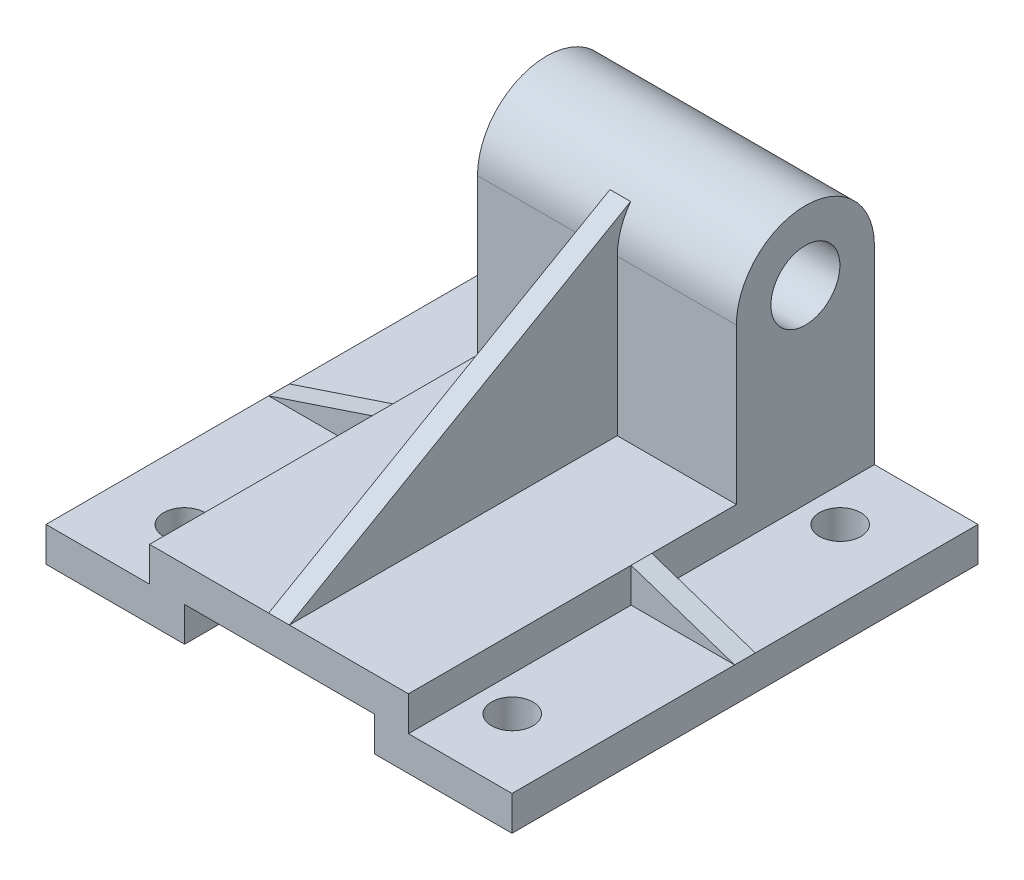
ISO-10303-21;
HEADER;
FILE_DESCRIPTION(('STEP AP214'),'2;1');
FILE_NAME('part.step','',(''),(''),'','','');
FILE_SCHEMA(('AUTOMOTIVE_DESIGN { 1 0 10303 214 1 1 1 1 }'));
ENDSEC;
DATA;
#1=APPLICATION_CONTEXT('core data for automotive mechanical design processes');
#2=APPLICATION_PROTOCOL_DEFINITION('international standard','automotive_design',2000,#1);
#3=PRODUCT_CONTEXT('',#1,'mechanical');
#4=PRODUCT('Part','Part','',(#3));
#5=PRODUCT_RELATED_PRODUCT_CATEGORY('part','',(#4));
#6=PRODUCT_DEFINITION_FORMATION('','',#4);
#7=PRODUCT_DEFINITION_CONTEXT('part definition',#1,'design');
#8=PRODUCT_DEFINITION('design','',#6,#7);
#9=PRODUCT_DEFINITION_SHAPE('','',#8);
#10=(LENGTH_UNIT() NAMED_UNIT(*) SI_UNIT(.MILLI.,.METRE.));
#11=(NAMED_UNIT(*) PLANE_ANGLE_UNIT() SI_UNIT($,.RADIAN.));
#12=(NAMED_UNIT(*) SI_UNIT($,.STERADIAN.) SOLID_ANGLE_UNIT());
#13=UNCERTAINTY_MEASURE_WITH_UNIT(LENGTH_MEASURE(1.E-05),#10,'distance_accuracy_value','');
#14=(GEOMETRIC_REPRESENTATION_CONTEXT(3) GLOBAL_UNCERTAINTY_ASSIGNED_CONTEXT((#13)) GLOBAL_UNIT_ASSIGNED_CONTEXT((#10,
#11,#12)) REPRESENTATION_CONTEXT('',''));
#15=CARTESIAN_POINT('',(0.,0.,0.));
#16=DIRECTION('',(0.,0.,1.));
#17=DIRECTION('',(1.,0.,0.));
#18=AXIS2_PLACEMENT_3D('',#15,#16,#17);
#19=CARTESIAN_POINT('',(-67.5,10.,67.5));
#20=DIRECTION('',(0.,-1.,0.));
#21=DIRECTION('',(0.,0.,-1.));
#22=AXIS2_PLACEMENT_3D('',#19,#20,#21);
#23=PLANE('',#22);
#24=DIRECTION('',(0.,0.,-1.));
#25=VECTOR('',#24,1.);
#26=CARTESIAN_POINT('',(-3.,10.,-35.5000326124525));
#27=LINE('',#26,#25);
#28=CARTESIAN_POINT('',(-3.,10.,67.5));
#29=VERTEX_POINT('',#28);
#30=CARTESIAN_POINT('',(-3.,10.,-27.5));
#31=VERTEX_POINT('',#30);
#32=EDGE_CURVE('E288',#29,#31,#27,.T.);
#33=ORIENTED_EDGE('',*,*,#32,.T.);
#34=DIRECTION('',(1.,0.,0.));
#35=VECTOR('',#34,1.);
#36=CARTESIAN_POINT('',(-37.5,10.,-27.5));
#37=LINE('',#36,#35);
#38=CARTESIAN_POINT('',(-37.5,10.,-27.5));
#39=VERTEX_POINT('',#38);
#40=EDGE_CURVE('E358',#39,#31,#37,.T.);
#41=ORIENTED_EDGE('',*,*,#40,.F.);
#42=DIRECTION('',(0.,0.,1.));
#43=VECTOR('',#42,1.);
#44=CARTESIAN_POINT('',(-37.5,10.,-67.5));
#45=LINE('',#44,#43);
#46=CARTESIAN_POINT('',(-37.5,10.,-3.));
#47=VERTEX_POINT('',#46);
#48=EDGE_CURVE('E382',#39,#47,#45,.T.);
#49=ORIENTED_EDGE('',*,*,#48,.T.);
#50=DIRECTION('',(0.,0.,-1.));
#51=VECTOR('',#50,1.);
#52=CARTESIAN_POINT('',(-37.5,10.,3.));
#53=LINE('',#52,#51);
#54=CARTESIAN_POINT('',(-37.5,10.,3.));
#55=VERTEX_POINT('',#54);
#56=EDGE_CURVE('E332',#55,#47,#53,.T.);
#57=ORIENTED_EDGE('',*,*,#56,.F.);
#58=CARTESIAN_POINT('',(-37.5,10.,67.5));
#59=VERTEX_POINT('',#58);
#60=EDGE_CURVE('E381',#55,#59,#45,.T.);
#61=ORIENTED_EDGE('',*,*,#60,.T.);
#62=DIRECTION('',(-1.,0.,0.));
#63=VECTOR('',#62,1.);
#64=CARTESIAN_POINT('',(-67.5,10.,67.5));
#65=LINE('',#64,#63);
#66=EDGE_CURVE('E232',#29,#59,#65,.T.);
#67=ORIENTED_EDGE('',*,*,#66,.F.);
#68=EDGE_LOOP('',(#33,#41,#49,#57,#61,#67));
#69=FACE_BOUND('',#68,.T.);
#70=ADVANCED_FACE('F41',(#69),#23,.F.);
#71=CARTESIAN_POINT('',(-37.5,55.,-27.5));
#72=DIRECTION('',(0.,0.,1.));
#73=DIRECTION('',(1.,0.,0.));
#74=AXIS2_PLACEMENT_3D('',#71,#72,#73);
#75=PLANE('',#74);
#76=ORIENTED_EDGE('',*,*,#40,.T.);
#77=DIRECTION('',(0.,1.,0.));
#78=VECTOR('',#77,1.);
#79=CARTESIAN_POINT('',(-3.,55.,-27.5));
#80=LINE('',#79,#78);
#81=CARTESIAN_POINT('',(-3.,55.,-27.5));
#82=VERTEX_POINT('',#81);
#83=EDGE_CURVE('E220',#31,#82,#80,.T.);
#84=ORIENTED_EDGE('',*,*,#83,.T.);
#85=DIRECTION('',(1.,0.,0.));
#86=VECTOR('',#85,1.);
#87=CARTESIAN_POINT('',(-37.5,55.,-27.5));
#88=LINE('',#87,#86);
#89=CARTESIAN_POINT('',(-37.5,55.,-27.5));
#90=VERTEX_POINT('',#89);
#91=EDGE_CURVE('E360',#90,#82,#88,.T.);
#92=ORIENTED_EDGE('',*,*,#91,.F.);
#93=DIRECTION('',(0.,-1.,0.));
#94=VECTOR('',#93,1.);
#95=CARTESIAN_POINT('',(-37.5,55.,-27.5));
#96=LINE('',#95,#94);
#97=EDGE_CURVE('E346',#90,#39,#96,.T.);
#98=ORIENTED_EDGE('',*,*,#97,.T.);
#99=EDGE_LOOP('',(#76,#84,#92,#98));
#100=FACE_BOUND('',#99,.T.);
#101=ADVANCED_FACE('F488',(#100),#75,.T.);
#102=CARTESIAN_POINT('',(37.5,0.,-67.5));
#103=DIRECTION('',(-1.,0.,0.));
#104=DIRECTION('',(0.,0.,1.));
#105=AXIS2_PLACEMENT_3D('',#102,#103,#104);
#106=PLANE('',#105);
#107=CARTESIAN_POINT('',(37.5,55.,-47.5));
#108=DIRECTION('',(1.,0.,0.));
#109=DIRECTION('',(0.,0.,-1.));
#110=AXIS2_PLACEMENT_3D('',#107,#108,#109);
#111=CIRCLE('',#110,10.);
#112=CARTESIAN_POINT('',(37.5,55.,-57.5));
#113=VERTEX_POINT('',#112);
#114=EDGE_CURVE('E340',#113,#113,#111,.T.);
#115=ORIENTED_EDGE('',*,*,#114,.F.);
#116=EDGE_LOOP('',(#115));
#117=FACE_BOUND('',#116,.T.);
#118=DIRECTION('',(0.,1.,0.));
#119=VECTOR('',#118,1.);
#120=CARTESIAN_POINT('',(37.5,10.,-3.));
#121=LINE('',#120,#119);
#122=CARTESIAN_POINT('',(37.5,0.,-3.));
#123=VERTEX_POINT('',#122);
#124=CARTESIAN_POINT('',(37.5,10.,-3.));
#125=VERTEX_POINT('',#124);
#126=EDGE_CURVE('E301',#123,#125,#121,.T.);
#127=ORIENTED_EDGE('',*,*,#126,.F.);
#128=DIRECTION('',(0.,0.,1.));
#129=VECTOR('',#128,1.);
#130=CARTESIAN_POINT('',(37.5,0.,-67.5));
#131=LINE('',#130,#129);
#132=CARTESIAN_POINT('',(37.5,0.,-67.5));
#133=VERTEX_POINT('',#132);
#134=EDGE_CURVE('E407',#133,#123,#131,.T.);
#135=ORIENTED_EDGE('',*,*,#134,.F.);
#136=DIRECTION('',(0.,-1.,0.));
#137=VECTOR('',#136,1.);
#138=CARTESIAN_POINT('',(37.5,0.,-67.5));
#139=LINE('',#138,#137);
#140=CARTESIAN_POINT('',(37.5,55.,-67.5));
#141=VERTEX_POINT('',#140);
#142=EDGE_CURVE('E389',#141,#133,#139,.T.);
#143=ORIENTED_EDGE('',*,*,#142,.F.);
#144=CARTESIAN_POINT('',(37.5,55.,-47.5));
#145=DIRECTION('',(1.,0.,0.));
#146=DIRECTION('',(0.,0.,-1.));
#147=AXIS2_PLACEMENT_3D('',#144,#145,#146);
#148=CIRCLE('',#147,20.);
#149=CARTESIAN_POINT('',(37.5,55.,-27.5));
#150=VERTEX_POINT('',#149);
#151=EDGE_CURVE('E342',#141,#150,#148,.T.);
#152=ORIENTED_EDGE('',*,*,#151,.T.);
#153=DIRECTION('',(0.,-1.,0.));
#154=VECTOR('',#153,1.);
#155=CARTESIAN_POINT('',(37.5,55.,-27.5));
#156=LINE('',#155,#154);
#157=CARTESIAN_POINT('',(37.5,10.,-27.5));
#158=VERTEX_POINT('',#157);
#159=EDGE_CURVE('E350',#150,#158,#156,.T.);
#160=ORIENTED_EDGE('',*,*,#159,.T.);
#161=DIRECTION('',(0.,0.,1.));
#162=VECTOR('',#161,1.);
#163=CARTESIAN_POINT('',(37.5,10.,-67.5));
#164=LINE('',#163,#162);
#165=EDGE_CURVE('E372',#158,#125,#164,.T.);
#166=ORIENTED_EDGE('',*,*,#165,.T.);
#167=EDGE_LOOP('',(#127,#135,#143,#152,#160,#166));
#168=FACE_BOUND('',#167,.T.);
#169=ADVANCED_FACE('F493',(#117,#168),#106,.F.);
#170=CARTESIAN_POINT('',(0.,0.,-67.5));
#171=DIRECTION('',(0.,-1.,0.));
#172=DIRECTION('',(0.,0.,-1.));
#173=AXIS2_PLACEMENT_3D('',#170,#171,#172);
#174=PLANE('',#173);
#175=CARTESIAN_POINT('',(47.5715920769878,0.,-47.5));
#176=DIRECTION('',(0.,-1.,0.));
#177=DIRECTION('',(0.,0.,-1.));
#178=AXIS2_PLACEMENT_3D('',#175,#176,#177);
#179=CIRCLE('',#178,6.);
#180=CARTESIAN_POINT('',(47.5715920769878,0.,-53.5));
#181=VERTEX_POINT('',#180);
#182=EDGE_CURVE('E286',#181,#181,#179,.T.);
#183=ORIENTED_EDGE('',*,*,#182,.T.);
#184=EDGE_LOOP('',(#183));
#185=FACE_BOUND('',#184,.T.);
#186=DIRECTION('',(-1.,0.,0.));
#187=VECTOR('',#186,1.);
#188=CARTESIAN_POINT('',(37.5,0.,-3.));
#189=LINE('',#188,#187);
#190=CARTESIAN_POINT('',(67.5000000000001,0.,-3.));
#191=VERTEX_POINT('',#190);
#192=EDGE_CURVE('E300',#191,#123,#189,.T.);
#193=ORIENTED_EDGE('',*,*,#192,.F.);
#194=DIRECTION('',(0.,0.,1.));
#195=VECTOR('',#194,1.);
#196=CARTESIAN_POINT('',(67.5000000000001,0.,-67.5));
#197=LINE('',#196,#195);
#198=CARTESIAN_POINT('',(67.5000000000001,0.,-67.5));
#199=VERTEX_POINT('',#198);
#200=EDGE_CURVE('E405',#199,#191,#197,.T.);
#201=ORIENTED_EDGE('',*,*,#200,.F.);
#202=DIRECTION('',(1.,0.,0.));
#203=VECTOR('',#202,1.);
#204=CARTESIAN_POINT('',(0.,0.,-67.5));
#205=LINE('',#204,#203);
#206=EDGE_CURVE('E394',#133,#199,#205,.T.);
#207=ORIENTED_EDGE('',*,*,#206,.F.);
#208=ORIENTED_EDGE('',*,*,#134,.T.);
#209=EDGE_LOOP('',(#193,#201,#207,#208));
#210=FACE_BOUND('',#209,.T.);
#211=ADVANCED_FACE('F514',(#185,#210),#174,.F.);
#212=CARTESIAN_POINT('',(0.,0.,-67.5));
#213=DIRECTION('',(0.,1.,0.));
#214=DIRECTION('',(0.,0.,1.));
#215=AXIS2_PLACEMENT_3D('',#212,#213,#214);
#216=PLANE('',#215);
#217=CARTESIAN_POINT('',(-47.4284079230122,0.,-47.5));
#218=DIRECTION('',(0.,1.,0.));
#219=DIRECTION('',(0.,0.,1.));
#220=AXIS2_PLACEMENT_3D('',#217,#218,#219);
#221=CIRCLE('',#220,6.);
#222=CARTESIAN_POINT('',(-47.4284079230122,0.,-41.5));
#223=VERTEX_POINT('',#222);
#224=EDGE_CURVE('E272',#223,#223,#221,.T.);
#225=ORIENTED_EDGE('',*,*,#224,.F.);
#226=EDGE_LOOP('',(#225));
#227=FACE_BOUND('',#226,.T.);
#228=DIRECTION('',(0.,0.,1.));
#229=VECTOR('',#228,1.);
#230=CARTESIAN_POINT('',(-67.5,0.,-67.5));
#231=LINE('',#230,#229);
#232=CARTESIAN_POINT('',(-67.5,0.,-67.5));
#233=VERTEX_POINT('',#232);
#234=CARTESIAN_POINT('',(-67.5,0.,-3.));
#235=VERTEX_POINT('',#234);
#236=EDGE_CURVE('E376',#233,#235,#231,.T.);
#237=ORIENTED_EDGE('',*,*,#236,.T.);
#238=DIRECTION('',(1.,0.,0.));
#239=VECTOR('',#238,1.);
#240=CARTESIAN_POINT('',(-37.5,0.,-3.));
#241=LINE('',#240,#239);
#242=CARTESIAN_POINT('',(-37.5,0.,-3.));
#243=VERTEX_POINT('',#242);
#244=EDGE_CURVE('E320',#235,#243,#241,.T.);
#245=ORIENTED_EDGE('',*,*,#244,.T.);
#246=DIRECTION('',(0.,0.,1.));
#247=VECTOR('',#246,1.);
#248=CARTESIAN_POINT('',(-37.5,0.,-67.5));
#249=LINE('',#248,#247);
#250=CARTESIAN_POINT('',(-37.5,0.,-67.5));
#251=VERTEX_POINT('',#250);
#252=EDGE_CURVE('E383',#251,#243,#249,.T.);
#253=ORIENTED_EDGE('',*,*,#252,.F.);
#254=DIRECTION('',(-1.,0.,0.));
#255=VECTOR('',#254,1.);
#256=CARTESIAN_POINT('',(0.,0.,-67.5));
#257=LINE('',#256,#255);
#258=EDGE_CURVE('E362',#251,#233,#257,.T.);
#259=ORIENTED_EDGE('',*,*,#258,.T.);
#260=EDGE_LOOP('',(#237,#245,#253,#259));
#261=FACE_BOUND('',#260,.T.);
#262=ADVANCED_FACE('F504',(#227,#261),#216,.T.);
#263=CARTESIAN_POINT('',(-37.5,0.,-67.5));
#264=DIRECTION('',(-1.,0.,0.));
#265=DIRECTION('',(0.,0.,1.));
#266=AXIS2_PLACEMENT_3D('',#263,#264,#265);
#267=PLANE('',#266);
#268=CARTESIAN_POINT('',(-37.5,55.,-47.5));
#269=DIRECTION('',(1.,0.,0.));
#270=DIRECTION('',(0.,0.,-1.));
#271=AXIS2_PLACEMENT_3D('',#268,#269,#270);
#272=CIRCLE('',#271,10.);
#273=CARTESIAN_POINT('',(-37.5,55.,-57.5));
#274=VERTEX_POINT('',#273);
#275=EDGE_CURVE('E336',#274,#274,#272,.T.);
#276=ORIENTED_EDGE('',*,*,#275,.T.);
#277=EDGE_LOOP('',(#276));
#278=FACE_BOUND('',#277,.T.);
#279=ORIENTED_EDGE('',*,*,#252,.T.);
#280=DIRECTION('',(0.,1.,0.));
#281=VECTOR('',#280,1.);
#282=CARTESIAN_POINT('',(-37.5,10.,-3.));
#283=LINE('',#282,#281);
#284=EDGE_CURVE('E330',#243,#47,#283,.T.);
#285=ORIENTED_EDGE('',*,*,#284,.T.);
#286=ORIENTED_EDGE('',*,*,#48,.F.);
#287=ORIENTED_EDGE('',*,*,#97,.F.);
#288=CARTESIAN_POINT('',(-37.5,55.,-47.5));
#289=DIRECTION('',(1.,0.,0.));
#290=DIRECTION('',(0.,0.,-1.));
#291=AXIS2_PLACEMENT_3D('',#288,#289,#290);
#292=CIRCLE('',#291,20.);
#293=CARTESIAN_POINT('',(-37.5,55.,-67.5));
#294=VERTEX_POINT('',#293);
#295=EDGE_CURVE('E341',#294,#90,#292,.T.);
#296=ORIENTED_EDGE('',*,*,#295,.F.);
#297=DIRECTION('',(0.,-1.,0.));
#298=VECTOR('',#297,1.);
#299=CARTESIAN_POINT('',(-37.5,0.,-67.5));
#300=LINE('',#299,#298);
#301=EDGE_CURVE('E370',#294,#251,#300,.T.);
#302=ORIENTED_EDGE('',*,*,#301,.T.);
#303=EDGE_LOOP('',(#279,#285,#286,#287,#296,#302));
#304=FACE_BOUND('',#303,.T.);
#305=ADVANCED_FACE('F498',(#278,#304),#267,.T.);
#306=CARTESIAN_POINT('',(3.,10.,-27.5));
#307=VERTEX_POINT('',#306);
#308=EDGE_CURVE('E228',#307,#158,#37,.T.);
#309=ORIENTED_EDGE('',*,*,#308,.F.);
#310=DIRECTION('',(0.,0.,-1.));
#311=VECTOR('',#310,1.);
#312=CARTESIAN_POINT('',(3.,10.,-29.4496870036438));
#313=LINE('',#312,#311);
#314=CARTESIAN_POINT('',(3.,10.,67.5));
#315=VERTEX_POINT('',#314);
#316=EDGE_CURVE('E210',#315,#307,#313,.T.);
#317=ORIENTED_EDGE('',*,*,#316,.F.);
#318=CARTESIAN_POINT('',(37.5,10.,67.5));
#319=VERTEX_POINT('',#318);
#320=EDGE_CURVE('E222',#319,#315,#65,.T.);
#321=ORIENTED_EDGE('',*,*,#320,.F.);
#322=CARTESIAN_POINT('',(37.5,10.,3.));
#323=VERTEX_POINT('',#322);
#324=EDGE_CURVE('E402',#323,#319,#164,.T.);
#325=ORIENTED_EDGE('',*,*,#324,.F.);
#326=DIRECTION('',(0.,0.,-1.));
#327=VECTOR('',#326,1.);
#328=CARTESIAN_POINT('',(37.5,10.,3.));
#329=LINE('',#328,#327);
#330=EDGE_CURVE('E304',#323,#125,#329,.T.);
#331=ORIENTED_EDGE('',*,*,#330,.T.);
#332=ORIENTED_EDGE('',*,*,#165,.F.);
#333=EDGE_LOOP('',(#309,#317,#321,#325,#331,#332));
#334=FACE_BOUND('',#333,.T.);
#335=ADVANCED_FACE('F223',(#334),#23,.F.);
#336=CARTESIAN_POINT('',(-67.5,10.,67.5));
#337=DIRECTION('',(1.,0.,0.));
#338=DIRECTION('',(0.,1.,0.));
#339=AXIS2_PLACEMENT_3D('',#336,#337,#338);
#340=PLANE('',#339);
#341=ORIENTED_EDGE('',*,*,#236,.F.);
#342=DIRECTION('',(0.,-1.,0.));
#343=VECTOR('',#342,1.);
#344=CARTESIAN_POINT('',(-67.5,10.,-67.5));
#345=LINE('',#344,#343);
#346=CARTESIAN_POINT('',(-67.4999999999999,-10.,-67.5));
#347=VERTEX_POINT('',#346);
#348=EDGE_CURVE('E249',#233,#347,#345,.T.);
#349=ORIENTED_EDGE('',*,*,#348,.T.);
#350=DIRECTION('',(0.,0.,-1.));
#351=VECTOR('',#350,1.);
#352=CARTESIAN_POINT('',(-67.4999999999999,-10.,67.5));
#353=LINE('',#352,#351);
#354=CARTESIAN_POINT('',(-67.4999999999999,-10.,67.5));
#355=VERTEX_POINT('',#354);
#356=EDGE_CURVE('E256',#355,#347,#353,.T.);
#357=ORIENTED_EDGE('',*,*,#356,.F.);
#358=DIRECTION('',(0.,-1.,0.));
#359=VECTOR('',#358,1.);
#360=CARTESIAN_POINT('',(-67.5,10.,67.5));
#361=LINE('',#360,#359);
#362=CARTESIAN_POINT('',(-67.5,0.,67.5));
#363=VERTEX_POINT('',#362);
#364=EDGE_CURVE('E234',#363,#355,#361,.T.);
#365=ORIENTED_EDGE('',*,*,#364,.F.);
#366=CARTESIAN_POINT('',(-67.5,0.,3.));
#367=VERTEX_POINT('',#366);
#368=EDGE_CURVE('E379',#367,#363,#231,.T.);
#369=ORIENTED_EDGE('',*,*,#368,.F.);
#370=DIRECTION('',(0.,0.,-1.));
#371=VECTOR('',#370,1.);
#372=CARTESIAN_POINT('',(-67.5,0.,3.));
#373=LINE('',#372,#371);
#374=EDGE_CURVE('E323',#367,#235,#373,.T.);
#375=ORIENTED_EDGE('',*,*,#374,.T.);
#376=EDGE_LOOP('',(#341,#349,#357,#365,#369,#375));
#377=FACE_BOUND('',#376,.T.);
#378=ADVANCED_FACE('F500',(#377),#340,.F.);
#379=CARTESIAN_POINT('',(0.,0.,67.5));
#380=DIRECTION('',(0.,0.,1.));
#381=DIRECTION('',(1.,0.,0.));
#382=AXIS2_PLACEMENT_3D('',#379,#380,#381);
#383=PLANE('',#382);
#384=DIRECTION('',(0.,-1.,0.));
#385=VECTOR('',#384,1.);
#386=CARTESIAN_POINT('',(-37.5,0.,67.5));
#387=LINE('',#386,#385);
#388=CARTESIAN_POINT('',(-37.5,0.,67.5));
#389=VERTEX_POINT('',#388);
#390=EDGE_CURVE('E368',#59,#389,#387,.T.);
#391=ORIENTED_EDGE('',*,*,#390,.T.);
#392=DIRECTION('',(-1.,0.,0.));
#393=VECTOR('',#392,1.);
#394=CARTESIAN_POINT('',(0.,0.,67.5));
#395=LINE('',#394,#393);
#396=EDGE_CURVE('E371',#389,#363,#395,.T.);
#397=ORIENTED_EDGE('',*,*,#396,.T.);
#398=ORIENTED_EDGE('',*,*,#364,.T.);
#399=DIRECTION('',(1.,0.,0.));
#400=VECTOR('',#399,1.);
#401=CARTESIAN_POINT('',(-67.4999999999999,-10.,67.5));
#402=LINE('',#401,#400);
#403=CARTESIAN_POINT('',(-27.3568158460245,-10.,67.5));
#404=VERTEX_POINT('',#403);
#405=EDGE_CURVE('E243',#355,#404,#402,.T.);
#406=ORIENTED_EDGE('',*,*,#405,.T.);
#407=DIRECTION('',(0.,-1.,0.));
#408=VECTOR('',#407,1.);
#409=CARTESIAN_POINT('',(-27.3568158460245,0.,67.5));
#410=LINE('',#409,#408);
#411=CARTESIAN_POINT('',(-27.3568158460245,0.,67.5));
#412=VERTEX_POINT('',#411);
#413=EDGE_CURVE('E378',#412,#404,#410,.T.);
#414=ORIENTED_EDGE('',*,*,#413,.F.);
#415=DIRECTION('',(-1.,0.,0.));
#416=VECTOR('',#415,1.);
#417=CARTESIAN_POINT('',(27.6431841539755,0.,67.5));
#418=LINE('',#417,#416);
#419=CARTESIAN_POINT('',(27.6431841539755,0.,67.5));
#420=VERTEX_POINT('',#419);
#421=EDGE_CURVE('E411',#420,#412,#418,.T.);
#422=ORIENTED_EDGE('',*,*,#421,.F.);
#423=DIRECTION('',(0.,1.,0.));
#424=VECTOR('',#423,1.);
#425=CARTESIAN_POINT('',(27.6431841539755,-10.,67.5));
#426=LINE('',#425,#424);
#427=CARTESIAN_POINT('',(27.6431841539755,-10.,67.5));
#428=VERTEX_POINT('',#427);
#429=EDGE_CURVE('E419',#428,#420,#426,.T.);
#430=ORIENTED_EDGE('',*,*,#429,.F.);
#431=CARTESIAN_POINT('',(67.5000000000001,-10.,67.5));
#432=VERTEX_POINT('',#431);
#433=EDGE_CURVE('E240',#428,#432,#402,.T.);
#434=ORIENTED_EDGE('',*,*,#433,.T.);
#435=DIRECTION('',(0.,1.,0.));
#436=VECTOR('',#435,1.);
#437=CARTESIAN_POINT('',(67.5000000000001,10.,67.5));
#438=LINE('',#437,#436);
#439=CARTESIAN_POINT('',(67.5000000000001,0.,67.5));
#440=VERTEX_POINT('',#439);
#441=EDGE_CURVE('E237',#432,#440,#438,.T.);
#442=ORIENTED_EDGE('',*,*,#441,.T.);
#443=DIRECTION('',(1.,0.,0.));
#444=VECTOR('',#443,1.);
#445=CARTESIAN_POINT('',(0.,0.,67.5));
#446=LINE('',#445,#444);
#447=CARTESIAN_POINT('',(37.5,0.,67.5));
#448=VERTEX_POINT('',#447);
#449=EDGE_CURVE('E391',#448,#440,#446,.T.);
#450=ORIENTED_EDGE('',*,*,#449,.F.);
#451=DIRECTION('',(0.,-1.,0.));
#452=VECTOR('',#451,1.);
#453=CARTESIAN_POINT('',(37.5,0.,67.5));
#454=LINE('',#453,#452);
#455=EDGE_CURVE('E231',#319,#448,#454,.T.);
#456=ORIENTED_EDGE('',*,*,#455,.F.);
#457=ORIENTED_EDGE('',*,*,#320,.T.);
#458=DIRECTION('',(-1.,0.,0.));
#459=VECTOR('',#458,1.);
#460=CARTESIAN_POINT('',(3.,10.,67.5));
#461=LINE('',#460,#459);
#462=EDGE_CURVE('E215',#315,#29,#461,.T.);
#463=ORIENTED_EDGE('',*,*,#462,.T.);
#464=ORIENTED_EDGE('',*,*,#66,.T.);
#465=EDGE_LOOP('',(#391,#397,#398,#406,#414,#422,#430,#434,#442,#450,#456,#457,#463,#464));
#466=FACE_BOUND('',#465,.T.);
#467=ADVANCED_FACE('F229',(#466),#383,.T.);
#468=CARTESIAN_POINT('',(0.,0.,-67.5));
#469=DIRECTION('',(0.,0.,1.));
#470=DIRECTION('',(1.,0.,0.));
#471=AXIS2_PLACEMENT_3D('',#468,#469,#470);
#472=PLANE('',#471);
#473=ORIENTED_EDGE('',*,*,#258,.F.);
#474=ORIENTED_EDGE('',*,*,#301,.F.);
#475=DIRECTION('',(1.,0.,0.));
#476=VECTOR('',#475,1.);
#477=CARTESIAN_POINT('',(-37.5,55.,-67.5));
#478=LINE('',#477,#476);
#479=EDGE_CURVE('E351',#294,#141,#478,.T.);
#480=ORIENTED_EDGE('',*,*,#479,.T.);
#481=ORIENTED_EDGE('',*,*,#142,.T.);
#482=ORIENTED_EDGE('',*,*,#206,.T.);
#483=DIRECTION('',(0.,1.,0.));
#484=VECTOR('',#483,1.);
#485=CARTESIAN_POINT('',(67.5000000000001,10.,-67.5));
#486=LINE('',#485,#484);
#487=CARTESIAN_POINT('',(67.5000000000001,-10.,-67.5));
#488=VERTEX_POINT('',#487);
#489=EDGE_CURVE('E250',#488,#199,#486,.T.);
#490=ORIENTED_EDGE('',*,*,#489,.F.);
#491=DIRECTION('',(1.,0.,0.));
#492=VECTOR('',#491,1.);
#493=CARTESIAN_POINT('',(-67.4999999999999,-10.,-67.5));
#494=LINE('',#493,#492);
#495=CARTESIAN_POINT('',(27.6431841539755,-10.,-67.5));
#496=VERTEX_POINT('',#495);
#497=EDGE_CURVE('E254',#496,#488,#494,.T.);
#498=ORIENTED_EDGE('',*,*,#497,.F.);
#499=DIRECTION('',(0.,1.,0.));
#500=VECTOR('',#499,1.);
#501=CARTESIAN_POINT('',(27.6431841539755,-10.,-67.5));
#502=LINE('',#501,#500);
#503=CARTESIAN_POINT('',(27.6431841539755,0.,-67.5));
#504=VERTEX_POINT('',#503);
#505=EDGE_CURVE('E412',#496,#504,#502,.T.);
#506=ORIENTED_EDGE('',*,*,#505,.T.);
#507=DIRECTION('',(-1.,0.,0.));
#508=VECTOR('',#507,1.);
#509=CARTESIAN_POINT('',(0.,0.,-67.5));
#510=LINE('',#509,#508);
#511=CARTESIAN_POINT('',(-27.3568158460245,0.,-67.5));
#512=VERTEX_POINT('',#511);
#513=EDGE_CURVE('E409',#504,#512,#510,.T.);
#514=ORIENTED_EDGE('',*,*,#513,.T.);
#515=DIRECTION('',(0.,-1.,0.));
#516=VECTOR('',#515,1.);
#517=CARTESIAN_POINT('',(-27.3568158460245,0.,-67.5));
#518=LINE('',#517,#516);
#519=CARTESIAN_POINT('',(-27.3568158460245,-10.,-67.5));
#520=VERTEX_POINT('',#519);
#521=EDGE_CURVE('E414',#512,#520,#518,.T.);
#522=ORIENTED_EDGE('',*,*,#521,.T.);
#523=EDGE_CURVE('E251',#347,#520,#494,.T.);
#524=ORIENTED_EDGE('',*,*,#523,.F.);
#525=ORIENTED_EDGE('',*,*,#348,.F.);
#526=EDGE_LOOP('',(#473,#474,#480,#481,#482,#490,#498,#506,#514,#522,#524,#525));
#527=FACE_BOUND('',#526,.T.);
#528=ADVANCED_FACE('F444',(#527),#472,.F.);
#529=CARTESIAN_POINT('',(-67.4999999999999,-10.,67.5));
#530=DIRECTION('',(0.,1.,0.));
#531=DIRECTION('',(0.,0.,1.));
#532=AXIS2_PLACEMENT_3D('',#529,#530,#531);
#533=PLANE('',#532);
#534=CARTESIAN_POINT('',(47.5715920769878,-10.,47.5));
#535=DIRECTION('',(0.,-1.,0.));
#536=DIRECTION('',(0.,0.,-1.));
#537=AXIS2_PLACEMENT_3D('',#534,#535,#536);
#538=CIRCLE('',#537,6.);
#539=CARTESIAN_POINT('',(47.5715920769878,-10.,41.5));
#540=VERTEX_POINT('',#539);
#541=EDGE_CURVE('E281',#540,#540,#538,.T.);
#542=ORIENTED_EDGE('',*,*,#541,.F.);
#543=EDGE_LOOP('',(#542));
#544=FACE_BOUND('',#543,.T.);
#545=CARTESIAN_POINT('',(47.5715920769878,-10.,-47.5));
#546=DIRECTION('',(0.,-1.,0.));
#547=DIRECTION('',(0.,0.,-1.));
#548=AXIS2_PLACEMENT_3D('',#545,#546,#547);
#549=CIRCLE('',#548,6.);
#550=CARTESIAN_POINT('',(47.5715920769878,-10.,-53.5));
#551=VERTEX_POINT('',#550);
#552=EDGE_CURVE('E270',#551,#551,#549,.T.);
#553=ORIENTED_EDGE('',*,*,#552,.F.);
#554=EDGE_LOOP('',(#553));
#555=FACE_BOUND('',#554,.T.);
#556=ORIENTED_EDGE('',*,*,#433,.F.);
#557=DIRECTION('',(0.,0.,1.));
#558=VECTOR('',#557,1.);
#559=CARTESIAN_POINT('',(27.6431841539755,-10.,-67.5));
#560=LINE('',#559,#558);
#561=EDGE_CURVE('E424',#496,#428,#560,.T.);
#562=ORIENTED_EDGE('',*,*,#561,.F.);
#563=ORIENTED_EDGE('',*,*,#497,.T.);
#564=DIRECTION('',(0.,0.,-1.));
#565=VECTOR('',#564,1.);
#566=CARTESIAN_POINT('',(67.5000000000001,-10.,67.5));
#567=LINE('',#566,#565);
#568=EDGE_CURVE('E246',#432,#488,#567,.T.);
#569=ORIENTED_EDGE('',*,*,#568,.F.);
#570=EDGE_LOOP('',(#556,#562,#563,#569));
#571=FACE_BOUND('',#570,.T.);
#572=ADVANCED_FACE('F456',(#544,#555,#571),#533,.F.);
#573=CARTESIAN_POINT('',(67.5000000000001,10.,67.5));
#574=DIRECTION('',(-1.,0.,0.));
#575=DIRECTION('',(0.,0.,1.));
#576=AXIS2_PLACEMENT_3D('',#573,#574,#575);
#577=PLANE('',#576);
#578=ORIENTED_EDGE('',*,*,#489,.T.);
#579=ORIENTED_EDGE('',*,*,#200,.T.);
#580=DIRECTION('',(0.,0.,-1.));
#581=VECTOR('',#580,1.);
#582=CARTESIAN_POINT('',(67.5,0.,3.));
#583=LINE('',#582,#581);
#584=CARTESIAN_POINT('',(67.5000000000001,0.,3.));
#585=VERTEX_POINT('',#584);
#586=EDGE_CURVE('E313',#585,#191,#583,.T.);
#587=ORIENTED_EDGE('',*,*,#586,.F.);
#588=EDGE_CURVE('E403',#585,#440,#197,.T.);
#589=ORIENTED_EDGE('',*,*,#588,.T.);
#590=ORIENTED_EDGE('',*,*,#441,.F.);
#591=ORIENTED_EDGE('',*,*,#568,.T.);
#592=EDGE_LOOP('',(#578,#579,#587,#589,#590,#591));
#593=FACE_BOUND('',#592,.T.);
#594=ADVANCED_FACE('F43',(#593),#577,.F.);
#595=CARTESIAN_POINT('',(-47.4284079230122,-10.,47.5));
#596=DIRECTION('',(0.,-1.,0.));
#597=DIRECTION('',(0.,0.,-1.));
#598=AXIS2_PLACEMENT_3D('',#595,#596,#597);
#599=CIRCLE('',#598,6.);
#600=CARTESIAN_POINT('',(-47.4284079230122,-10.,41.5));
#601=VERTEX_POINT('',#600);
#602=EDGE_CURVE('E279',#601,#601,#599,.T.);
#603=ORIENTED_EDGE('',*,*,#602,.F.);
#604=EDGE_LOOP('',(#603));
#605=FACE_BOUND('',#604,.T.);
#606=CARTESIAN_POINT('',(-47.4284079230122,-10.,-47.5));
#607=DIRECTION('',(0.,-1.,0.));
#608=DIRECTION('',(0.,0.,-1.));
#609=AXIS2_PLACEMENT_3D('',#606,#607,#608);
#610=CIRCLE('',#609,6.);
#611=CARTESIAN_POINT('',(-47.4284079230122,-10.,-53.5));
#612=VERTEX_POINT('',#611);
#613=EDGE_CURVE('E271',#612,#612,#610,.T.);
#614=ORIENTED_EDGE('',*,*,#613,.F.);
#615=EDGE_LOOP('',(#614));
#616=FACE_BOUND('',#615,.T.);
#617=ORIENTED_EDGE('',*,*,#523,.T.);
#618=DIRECTION('',(0.,0.,1.));
#619=VECTOR('',#618,1.);
#620=CARTESIAN_POINT('',(-27.3568158460245,-10.,-67.5));
#621=LINE('',#620,#619);
#622=EDGE_CURVE('E430',#520,#404,#621,.T.);
#623=ORIENTED_EDGE('',*,*,#622,.T.);
#624=ORIENTED_EDGE('',*,*,#405,.F.);
#625=ORIENTED_EDGE('',*,*,#356,.T.);
#626=EDGE_LOOP('',(#617,#623,#624,#625));
#627=FACE_BOUND('',#626,.T.);
#628=ADVANCED_FACE('F441',(#605,#616,#627),#533,.F.);
#629=CARTESIAN_POINT('',(27.6431841539755,0.,-67.5));
#630=DIRECTION('',(0.,1.,0.));
#631=DIRECTION('',(-1.,0.,0.));
#632=AXIS2_PLACEMENT_3D('',#629,#630,#631);
#633=PLANE('',#632);
#634=ORIENTED_EDGE('',*,*,#421,.T.);
#635=DIRECTION('',(0.,0.,1.));
#636=VECTOR('',#635,1.);
#637=CARTESIAN_POINT('',(-27.3568158460245,0.,-67.5));
#638=LINE('',#637,#636);
#639=EDGE_CURVE('E418',#512,#412,#638,.T.);
#640=ORIENTED_EDGE('',*,*,#639,.F.);
#641=ORIENTED_EDGE('',*,*,#513,.F.);
#642=DIRECTION('',(0.,0.,1.));
#643=VECTOR('',#642,1.);
#644=CARTESIAN_POINT('',(27.6431841539755,0.,-67.5));
#645=LINE('',#644,#643);
#646=EDGE_CURVE('E252',#504,#420,#645,.T.);
#647=ORIENTED_EDGE('',*,*,#646,.T.);
#648=EDGE_LOOP('',(#634,#640,#641,#647));
#649=FACE_BOUND('',#648,.T.);
#650=ADVANCED_FACE('F446',(#649),#633,.F.);
#651=CARTESIAN_POINT('',(27.6431841539755,-10.,-67.5));
#652=DIRECTION('',(1.,0.,0.));
#653=DIRECTION('',(0.,1.,0.));
#654=AXIS2_PLACEMENT_3D('',#651,#652,#653);
#655=PLANE('',#654);
#656=ORIENTED_EDGE('',*,*,#429,.T.);
#657=ORIENTED_EDGE('',*,*,#646,.F.);
#658=ORIENTED_EDGE('',*,*,#505,.F.);
#659=ORIENTED_EDGE('',*,*,#561,.T.);
#660=EDGE_LOOP('',(#656,#657,#658,#659));
#661=FACE_BOUND('',#660,.T.);
#662=ADVANCED_FACE('F452',(#661),#655,.F.);
#663=CARTESIAN_POINT('',(-27.3568158460245,0.,-67.5));
#664=DIRECTION('',(-1.,0.,0.));
#665=DIRECTION('',(0.,0.,1.));
#666=AXIS2_PLACEMENT_3D('',#663,#664,#665);
#667=PLANE('',#666);
#668=ORIENTED_EDGE('',*,*,#413,.T.);
#669=ORIENTED_EDGE('',*,*,#622,.F.);
#670=ORIENTED_EDGE('',*,*,#521,.F.);
#671=ORIENTED_EDGE('',*,*,#639,.T.);
#672=EDGE_LOOP('',(#668,#669,#670,#671));
#673=FACE_BOUND('',#672,.T.);
#674=ADVANCED_FACE('F433',(#673),#667,.F.);
#675=CARTESIAN_POINT('',(37.5,0.,3.));
#676=VERTEX_POINT('',#675);
#677=EDGE_CURVE('E392',#676,#448,#131,.T.);
#678=ORIENTED_EDGE('',*,*,#677,.F.);
#679=DIRECTION('',(0.,1.,0.));
#680=VECTOR('',#679,1.);
#681=CARTESIAN_POINT('',(37.5,10.,3.));
#682=LINE('',#681,#680);
#683=EDGE_CURVE('E69',#676,#323,#682,.T.);
#684=ORIENTED_EDGE('',*,*,#683,.T.);
#685=ORIENTED_EDGE('',*,*,#324,.T.);
#686=ORIENTED_EDGE('',*,*,#455,.T.);
#687=EDGE_LOOP('',(#678,#684,#685,#686));
#688=FACE_BOUND('',#687,.T.);
#689=ADVANCED_FACE('F464',(#688),#106,.F.);
#690=CARTESIAN_POINT('',(47.5715920769878,0.,47.5));
#691=DIRECTION('',(0.,-1.,0.));
#692=DIRECTION('',(0.,0.,-1.));
#693=AXIS2_PLACEMENT_3D('',#690,#691,#692);
#694=CIRCLE('',#693,6.);
#695=CARTESIAN_POINT('',(47.5715920769878,0.,41.5));
#696=VERTEX_POINT('',#695);
#697=EDGE_CURVE('E44',#696,#696,#694,.T.);
#698=ORIENTED_EDGE('',*,*,#697,.T.);
#699=EDGE_LOOP('',(#698));
#700=FACE_BOUND('',#699,.T.);
#701=ORIENTED_EDGE('',*,*,#588,.F.);
#702=DIRECTION('',(-1.,0.,0.));
#703=VECTOR('',#702,1.);
#704=CARTESIAN_POINT('',(37.5,0.,3.));
#705=LINE('',#704,#703);
#706=EDGE_CURVE('E296',#585,#676,#705,.T.);
#707=ORIENTED_EDGE('',*,*,#706,.T.);
#708=ORIENTED_EDGE('',*,*,#677,.T.);
#709=ORIENTED_EDGE('',*,*,#449,.T.);
#710=EDGE_LOOP('',(#701,#707,#708,#709));
#711=FACE_BOUND('',#710,.T.);
#712=ADVANCED_FACE('F463',(#700,#711),#174,.F.);
#713=CARTESIAN_POINT('',(-47.4284079230122,0.,47.5));
#714=DIRECTION('',(0.,1.,0.));
#715=DIRECTION('',(0.,0.,1.));
#716=AXIS2_PLACEMENT_3D('',#713,#714,#715);
#717=CIRCLE('',#716,6.);
#718=CARTESIAN_POINT('',(-47.4284079230122,0.,53.5));
#719=VERTEX_POINT('',#718);
#720=EDGE_CURVE('E262',#719,#719,#717,.T.);
#721=ORIENTED_EDGE('',*,*,#720,.F.);
#722=EDGE_LOOP('',(#721));
#723=FACE_BOUND('',#722,.T.);
#724=DIRECTION('',(1.,0.,0.));
#725=VECTOR('',#724,1.);
#726=CARTESIAN_POINT('',(-37.5,0.,3.));
#727=LINE('',#726,#725);
#728=CARTESIAN_POINT('',(-37.5,0.,3.));
#729=VERTEX_POINT('',#728);
#730=EDGE_CURVE('E319',#367,#729,#727,.T.);
#731=ORIENTED_EDGE('',*,*,#730,.F.);
#732=ORIENTED_EDGE('',*,*,#368,.T.);
#733=ORIENTED_EDGE('',*,*,#396,.F.);
#734=EDGE_CURVE('E369',#729,#389,#249,.T.);
#735=ORIENTED_EDGE('',*,*,#734,.F.);
#736=EDGE_LOOP('',(#731,#732,#733,#735));
#737=FACE_BOUND('',#736,.T.);
#738=ADVANCED_FACE('F517',(#723,#737),#216,.T.);
#739=DIRECTION('',(0.,1.,0.));
#740=VECTOR('',#739,1.);
#741=CARTESIAN_POINT('',(-37.5,10.,3.));
#742=LINE('',#741,#740);
#743=EDGE_CURVE('E318',#729,#55,#742,.T.);
#744=ORIENTED_EDGE('',*,*,#743,.F.);
#745=ORIENTED_EDGE('',*,*,#734,.T.);
#746=ORIENTED_EDGE('',*,*,#390,.F.);
#747=ORIENTED_EDGE('',*,*,#60,.F.);
#748=EDGE_LOOP('',(#744,#745,#746,#747));
#749=FACE_BOUND('',#748,.T.);
#750=ADVANCED_FACE('F507',(#749),#267,.T.);
#751=DIRECTION('',(0.,1.,0.));
#752=VECTOR('',#751,1.);
#753=CARTESIAN_POINT('',(3.,55.,-27.5));
#754=LINE('',#753,#752);
#755=CARTESIAN_POINT('',(3.,55.,-27.5));
#756=VERTEX_POINT('',#755);
#757=EDGE_CURVE('E294',#307,#756,#754,.T.);
#758=ORIENTED_EDGE('',*,*,#757,.F.);
#759=ORIENTED_EDGE('',*,*,#308,.T.);
#760=ORIENTED_EDGE('',*,*,#159,.F.);
#761=EDGE_CURVE('E365',#756,#150,#88,.T.);
#762=ORIENTED_EDGE('',*,*,#761,.F.);
#763=EDGE_LOOP('',(#758,#759,#760,#762));
#764=FACE_BOUND('',#763,.T.);
#765=ADVANCED_FACE('F494',(#764),#75,.T.);
#766=CARTESIAN_POINT('',(-37.5,55.,-47.5));
#767=DIRECTION('',(1.,0.,0.));
#768=DIRECTION('',(0.,0.,-1.));
#769=AXIS2_PLACEMENT_3D('',#766,#767,#768);
#770=CYLINDRICAL_SURFACE('',#769,20.);
#771=CARTESIAN_POINT('',(3.,55.,-47.5));
#772=DIRECTION('',(1.,0.,0.));
#773=DIRECTION('',(0.,0.,-1.));
#774=AXIS2_PLACEMENT_3D('',#771,#772,#773);
#775=CIRCLE('',#774,20.);
#776=CARTESIAN_POINT('',(3.,66.8240490784258,-31.3695361693788));
#777=VERTEX_POINT('',#776);
#778=EDGE_CURVE('E11',#756,#777,#775,.F.);
#779=ORIENTED_EDGE('',*,*,#778,.F.);
#780=ORIENTED_EDGE('',*,*,#761,.T.);
#781=ORIENTED_EDGE('',*,*,#151,.F.);
#782=ORIENTED_EDGE('',*,*,#479,.F.);
#783=ORIENTED_EDGE('',*,*,#295,.T.);
#784=ORIENTED_EDGE('',*,*,#91,.T.);
#785=CARTESIAN_POINT('',(-3.,55.,-47.5));
#786=DIRECTION('',(1.,0.,0.));
#787=DIRECTION('',(0.,0.,-1.));
#788=AXIS2_PLACEMENT_3D('',#785,#786,#787);
#789=CIRCLE('',#788,20.);
#790=CARTESIAN_POINT('',(-3.,66.8240490784258,-31.3695361693788));
#791=VERTEX_POINT('',#790);
#792=EDGE_CURVE('E261',#82,#791,#789,.F.);
#793=ORIENTED_EDGE('',*,*,#792,.T.);
#794=DIRECTION('',(1.,0.,0.));
#795=VECTOR('',#794,1.);
#796=CARTESIAN_POINT('',(-37.5,66.8240490784258,-31.3695361693788));
#797=LINE('',#796,#795);
#798=EDGE_CURVE('E49',#791,#777,#797,.T.);
#799=ORIENTED_EDGE('',*,*,#798,.T.);
#800=EDGE_LOOP('',(#779,#780,#781,#782,#783,#784,#793,#799));
#801=FACE_BOUND('',#800,.T.);
#802=ADVANCED_FACE('F522',(#801),#770,.T.);
#803=CARTESIAN_POINT('',(-37.5,55.,-47.5));
#804=DIRECTION('',(1.,0.,0.));
#805=DIRECTION('',(0.,0.,-1.));
#806=AXIS2_PLACEMENT_3D('',#803,#804,#805);
#807=CYLINDRICAL_SURFACE('',#806,10.);
#808=ORIENTED_EDGE('',*,*,#275,.F.);
#809=EDGE_LOOP('',(#808));
#810=FACE_BOUND('',#809,.T.);
#811=ORIENTED_EDGE('',*,*,#114,.T.);
#812=EDGE_LOOP('',(#811));
#813=FACE_BOUND('',#812,.T.);
#814=ADVANCED_FACE('F740',(#810,#813),#807,.F.);
#815=CARTESIAN_POINT('',(-67.5,0.,3.));
#816=DIRECTION('',(0.316227766016839,-0.948683298050514,0.));
#817=DIRECTION('',(0.948683298050514,0.316227766016839,0.));
#818=AXIS2_PLACEMENT_3D('',#815,#816,#817);
#819=PLANE('',#818);
#820=DIRECTION('',(-0.948683298050514,-0.316227766016839,0.));
#821=VECTOR('',#820,1.);
#822=CARTESIAN_POINT('',(-67.5,0.,-3.));
#823=LINE('',#822,#821);
#824=EDGE_CURVE('E322',#47,#235,#823,.T.);
#825=ORIENTED_EDGE('',*,*,#824,.T.);
#826=ORIENTED_EDGE('',*,*,#374,.F.);
#827=DIRECTION('',(-0.948683298050514,-0.316227766016839,0.));
#828=VECTOR('',#827,1.);
#829=CARTESIAN_POINT('',(-67.5,0.,3.));
#830=LINE('',#829,#828);
#831=EDGE_CURVE('E324',#55,#367,#830,.T.);
#832=ORIENTED_EDGE('',*,*,#831,.F.);
#833=ORIENTED_EDGE('',*,*,#56,.T.);
#834=EDGE_LOOP('',(#825,#826,#832,#833));
#835=FACE_BOUND('',#834,.T.);
#836=ADVANCED_FACE('F543',(#835),#819,.F.);
#837=CARTESIAN_POINT('',(0.,0.,3.));
#838=DIRECTION('',(0.,0.,1.));
#839=DIRECTION('',(1.,0.,0.));
#840=AXIS2_PLACEMENT_3D('',#837,#838,#839);
#841=PLANE('',#840);
#842=ORIENTED_EDGE('',*,*,#730,.T.);
#843=ORIENTED_EDGE('',*,*,#743,.T.);
#844=ORIENTED_EDGE('',*,*,#831,.T.);
#845=EDGE_LOOP('',(#842,#843,#844));
#846=FACE_BOUND('',#845,.T.);
#847=ADVANCED_FACE('F727',(#846),#841,.T.);
#848=CARTESIAN_POINT('',(0.,0.,-3.));
#849=DIRECTION('',(0.,0.,1.));
#850=DIRECTION('',(1.,0.,0.));
#851=AXIS2_PLACEMENT_3D('',#848,#849,#850);
#852=PLANE('',#851);
#853=ORIENTED_EDGE('',*,*,#244,.F.);
#854=ORIENTED_EDGE('',*,*,#824,.F.);
#855=ORIENTED_EDGE('',*,*,#284,.F.);
#856=EDGE_LOOP('',(#853,#854,#855));
#857=FACE_BOUND('',#856,.T.);
#858=ADVANCED_FACE('F485',(#857),#852,.F.);
#859=CARTESIAN_POINT('',(67.5,0.,3.));
#860=DIRECTION('',(0.316227766016839,0.948683298050514,0.));
#861=DIRECTION('',(-0.948683298050514,0.316227766016839,0.));
#862=AXIS2_PLACEMENT_3D('',#859,#860,#861);
#863=PLANE('',#862);
#864=DIRECTION('',(0.948683298050514,-0.316227766016839,0.));
#865=VECTOR('',#864,1.);
#866=CARTESIAN_POINT('',(67.5,0.,-3.));
#867=LINE('',#866,#865);
#868=EDGE_CURVE('E308',#125,#191,#867,.T.);
#869=ORIENTED_EDGE('',*,*,#868,.F.);
#870=ORIENTED_EDGE('',*,*,#330,.F.);
#871=DIRECTION('',(0.948683298050514,-0.316227766016839,0.));
#872=VECTOR('',#871,1.);
#873=CARTESIAN_POINT('',(67.5,0.,3.));
#874=LINE('',#873,#872);
#875=EDGE_CURVE('E297',#323,#585,#874,.T.);
#876=ORIENTED_EDGE('',*,*,#875,.T.);
#877=ORIENTED_EDGE('',*,*,#586,.T.);
#878=EDGE_LOOP('',(#869,#870,#876,#877));
#879=FACE_BOUND('',#878,.T.);
#880=ADVANCED_FACE('F468',(#879),#863,.T.);
#881=CARTESIAN_POINT('',(0.,0.,3.));
#882=DIRECTION('',(0.,0.,1.));
#883=DIRECTION('',(-1.,0.,0.));
#884=AXIS2_PLACEMENT_3D('',#881,#882,#883);
#885=PLANE('',#884);
#886=ORIENTED_EDGE('',*,*,#706,.F.);
#887=ORIENTED_EDGE('',*,*,#875,.F.);
#888=ORIENTED_EDGE('',*,*,#683,.F.);
#889=EDGE_LOOP('',(#886,#887,#888));
#890=FACE_BOUND('',#889,.T.);
#891=ADVANCED_FACE('F475',(#890),#885,.T.);
#892=CARTESIAN_POINT('',(0.,0.,-3.));
#893=DIRECTION('',(0.,0.,1.));
#894=DIRECTION('',(-1.,0.,0.));
#895=AXIS2_PLACEMENT_3D('',#892,#893,#894);
#896=PLANE('',#895);
#897=ORIENTED_EDGE('',*,*,#192,.T.);
#898=ORIENTED_EDGE('',*,*,#126,.T.);
#899=ORIENTED_EDGE('',*,*,#868,.T.);
#900=EDGE_LOOP('',(#897,#898,#899));
#901=FACE_BOUND('',#900,.T.);
#902=ADVANCED_FACE('F471',(#901),#896,.F.);
#903=CARTESIAN_POINT('',(3.,10.,67.5));
#904=DIRECTION('',(0.,-0.867004561474749,-0.498300201065561));
#905=DIRECTION('',(0.,0.498300201065561,-0.867004561474749));
#906=AXIS2_PLACEMENT_3D('',#903,#904,#905);
#907=PLANE('',#906);
#908=ORIENTED_EDGE('',*,*,#798,.F.);
#909=DIRECTION('',(0.,-0.498300201065561,0.867004561474749));
#910=VECTOR('',#909,1.);
#911=CARTESIAN_POINT('',(-3.,10.,67.5));
#912=LINE('',#911,#910);
#913=EDGE_CURVE('E59',#791,#29,#912,.T.);
#914=ORIENTED_EDGE('',*,*,#913,.T.);
#915=ORIENTED_EDGE('',*,*,#462,.F.);
#916=DIRECTION('',(0.,-0.498300201065561,0.867004561474749));
#917=VECTOR('',#916,1.);
#918=CARTESIAN_POINT('',(3.,10.,67.5));
#919=LINE('',#918,#917);
#920=EDGE_CURVE('E203',#777,#315,#919,.T.);
#921=ORIENTED_EDGE('',*,*,#920,.F.);
#922=EDGE_LOOP('',(#908,#914,#915,#921));
#923=FACE_BOUND('',#922,.T.);
#924=ADVANCED_FACE('F213',(#923),#907,.F.);
#925=CARTESIAN_POINT('',(3.,0.,0.));
#926=DIRECTION('',(1.,0.,0.));
#927=DIRECTION('',(0.,0.,-1.));
#928=AXIS2_PLACEMENT_3D('',#925,#926,#927);
#929=PLANE('',#928);
#930=ORIENTED_EDGE('',*,*,#316,.T.);
#931=ORIENTED_EDGE('',*,*,#757,.T.);
#932=ORIENTED_EDGE('',*,*,#778,.T.);
#933=ORIENTED_EDGE('',*,*,#920,.T.);
#934=EDGE_LOOP('',(#930,#931,#932,#933));
#935=FACE_BOUND('',#934,.T.);
#936=ADVANCED_FACE('F204',(#935),#929,.T.);
#937=CARTESIAN_POINT('',(-3.,0.,0.));
#938=DIRECTION('',(1.,0.,0.));
#939=DIRECTION('',(0.,0.,-1.));
#940=AXIS2_PLACEMENT_3D('',#937,#938,#939);
#941=PLANE('',#940);
#942=ORIENTED_EDGE('',*,*,#83,.F.);
#943=ORIENTED_EDGE('',*,*,#32,.F.);
#944=ORIENTED_EDGE('',*,*,#913,.F.);
#945=ORIENTED_EDGE('',*,*,#792,.F.);
#946=EDGE_LOOP('',(#942,#943,#944,#945));
#947=FACE_BOUND('',#946,.T.);
#948=ADVANCED_FACE('F558',(#947),#941,.F.);
#949=CARTESIAN_POINT('',(-47.4284079230122,75.,47.5));
#950=DIRECTION('',(0.,-1.,0.));
#951=DIRECTION('',(0.,0.,-1.));
#952=AXIS2_PLACEMENT_3D('',#949,#950,#951);
#953=CYLINDRICAL_SURFACE('',#952,6.);
#954=ORIENTED_EDGE('',*,*,#720,.T.);
#955=EDGE_LOOP('',(#954));
#956=FACE_BOUND('',#955,.T.);
#957=ORIENTED_EDGE('',*,*,#602,.T.);
#958=EDGE_LOOP('',(#957));
#959=FACE_BOUND('',#958,.T.);
#960=ADVANCED_FACE('F556',(#956,#959),#953,.F.);
#961=CARTESIAN_POINT('',(47.5715920769878,75.,47.5));
#962=DIRECTION('',(0.,-1.,0.));
#963=DIRECTION('',(0.,0.,-1.));
#964=AXIS2_PLACEMENT_3D('',#961,#962,#963);
#965=CYLINDRICAL_SURFACE('',#964,6.);
#966=ORIENTED_EDGE('',*,*,#541,.T.);
#967=EDGE_LOOP('',(#966));
#968=FACE_BOUND('',#967,.T.);
#969=ORIENTED_EDGE('',*,*,#697,.F.);
#970=EDGE_LOOP('',(#969));
#971=FACE_BOUND('',#970,.T.);
#972=ADVANCED_FACE('F564',(#968,#971),#965,.F.);
#973=CARTESIAN_POINT('',(-47.4284079230122,75.,-47.5));
#974=DIRECTION('',(0.,-1.,0.));
#975=DIRECTION('',(0.,0.,-1.));
#976=AXIS2_PLACEMENT_3D('',#973,#974,#975);
#977=CYLINDRICAL_SURFACE('',#976,6.);
#978=ORIENTED_EDGE('',*,*,#224,.T.);
#979=EDGE_LOOP('',(#978));
#980=FACE_BOUND('',#979,.T.);
#981=ORIENTED_EDGE('',*,*,#613,.T.);
#982=EDGE_LOOP('',(#981));
#983=FACE_BOUND('',#982,.T.);
#984=ADVANCED_FACE('F602',(#980,#983),#977,.F.);
#985=CARTESIAN_POINT('',(47.5715920769878,75.,-47.5));
#986=DIRECTION('',(0.,-1.,0.));
#987=DIRECTION('',(0.,0.,-1.));
#988=AXIS2_PLACEMENT_3D('',#985,#986,#987);
#989=CYLINDRICAL_SURFACE('',#988,6.);
#990=ORIENTED_EDGE('',*,*,#552,.T.);
#991=EDGE_LOOP('',(#990));
#992=FACE_BOUND('',#991,.T.);
#993=ORIENTED_EDGE('',*,*,#182,.F.);
#994=EDGE_LOOP('',(#993));
#995=FACE_BOUND('',#994,.T.);
#996=ADVANCED_FACE('F611',(#992,#995),#989,.F.);
#997=CLOSED_SHELL('',(#70,#101,#169,#211,#262,#305,#335,#378,#467,#528,#572,#594,#628,#650,#662,
#674,#689,#712,#738,#750,#765,#802,#814,#836,#847,#858,#880,#891,#902,#924,#936,#948,#960,#972,
#984,#996));
#998=MANIFOLD_SOLID_BREP('B2',#997);
#999=ADVANCED_BREP_SHAPE_REPRESENTATION('',(#18,#998),#14);
#1000=SHAPE_DEFINITION_REPRESENTATION(#9,#999);
ENDSEC;
END-ISO-10303-21;
